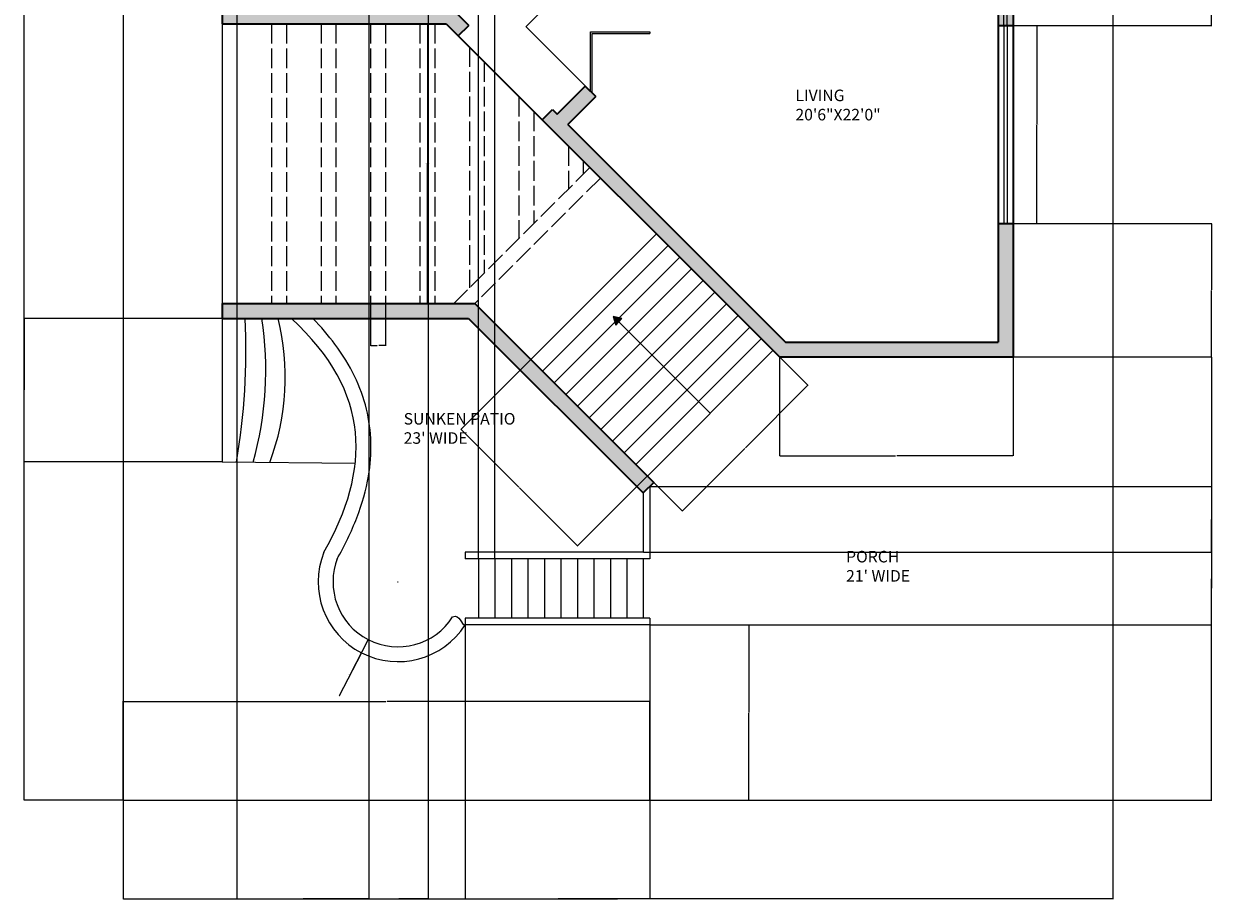
# Model space of a CAD drawing. Units: inches. Extents: x 1516 to 2236, y 3034 to 4235.
# Tile 1 of 3: x 1516 to 2236, y 3034 to 3566. Entities that reach past the tile are written whole.
import ezdxf

# ---------------------------------------------------------------- set-up
doc = ezdxf.new("R2010")
doc.units = ezdxf.units.IN
doc.linetypes.add('ACAD_ISO02W100', pattern=[15, 12, -3])
for name, color, linetype, lineweight in [('A-ANNO-DIMS', 2, 'Continuous', 18), ('A-ANNO-SYMB', 7, 'Continuous', 18), ('A-AREA-IDEN', 7, 'Continuous', 18), ('A-DOOR', 3, 'Continuous', 18), ('A-FLOR-STRS', 7, 'Continuous', 18), ('A-GLAZ', 4, 'Continuous', 18), ('A-ROOF-OVHD', 8, 'ACAD_ISO02W100', 18), ('A-WALL', 7, 'Continuous', 35), ('A-WALL-PATT', 252, 'Continuous', 13), ('C-PROP', 8, 'Continuous', 25), ('L-HRDS', 9, 'Continuous', 25)]:
    doc.layers.add(name, color=color, linetype=linetype, lineweight=lineweight)
doc.styles.get("Standard").update_dxf_attribs({"font": 'arial.ttf'})
doc.dimstyles.get("Standard").update_dxf_attribs({"dimtxt": 0.18, "dimasz": 0.18, "dimexe": 0.18, "dimexo": 0.0625, "dimgap": 0.09, "dimtad": 0, "dimtih": 1, "dimtoh": 1, "dimdec": 4, "dimzin": 0, "dimdsep": 46, "dimtxsty": 'Standard', "dimcen": 0.09, "dimadec": 0, "dimazin": 0, "dimtfac": 1, "dimtdec": 4, "dimtofl": 0, "dimtmove": 0, "dimatfit": 3, "dimfxl": 1, "dimtolj": 1, "dimtzin": 0, "dimarcsym": 0})

# ---------------------------------------------------------------- blocks, each defined once
blk = doc.blocks.new('WIN-120IN-GLASS')
for p, q in [((120, 2), (0, 2)), ((120, 0), (0, 0))]:
    blk.add_line(p, q)
blk = doc.blocks.new('TERRACE-OVHD-MEMBER')
for p, q in [((0, 169.71), (0, 0)), ((9, 169.71), (9, 0))]:
    blk.add_line(p, q)
blk = doc.blocks.new('*D10')
at = {"layer": 'A-ANNO-DIMS', "color": 0, "lineweight": -2, "transparency": 16777216}
for p, q in [((1735.08, 3565.52), (1760.65, 3565.52)), ((1760.47, 3565.34), (1760.47, 3480.85)), ((1760.47, 3396), (1760.47, 3480.49)), ((1735.08, 3395.82), (1760.65, 3395.82))]:
    blk.add_line(p, q, dxfattribs=at)
at = {"layer": 'A-ANNO-DIMS', "color": 0, "transparency": 16777216}
for points in [[(1760.44, 3565.34), (1760.5, 3565.34), (1760.47, 3565.52)], [(1760.44, 3396), (1760.5, 3396), (1760.47, 3395.82)]]:
    blk.add_solid(points, dxfattribs=at)
at = {"layer": 'Defpoints', "color": 0, "transparency": 16777216}
for p in [(1735.01, 3565.52), (1760.47, 3565.52), (1735.01, 3395.82)]:
    blk.add_point(p, dxfattribs=at)
at = {"layer": 'A-ANNO-DIMS', "color": 0, "transparency": 16777216, "insert": (1760.47, 3480.67), "char_height": 0.18, "attachment_point": 5}
blk.add_mtext('\\A1;OH MEMBER 170 TYP.', dxfattribs=at)
blk = doc.blocks.new('*D11')
at = {"layer": 'A-ANNO-DIMS', "color": 0, "lineweight": -2, "transparency": 16777216}
for p, q in [((1726.01, 3395.75), (1726.01, 3370.18)), ((1735.01, 3395.75), (1735.01, 3370.18)), ((1726.19, 3370.36), (1730.06, 3370.36)), ((1734.83, 3370.36), (1730.97, 3370.36))]:
    blk.add_line(p, q, dxfattribs=at)
at = {"layer": 'A-ANNO-DIMS', "color": 0, "transparency": 16777216}
for points in [[(1726.19, 3370.39), (1726.19, 3370.33), (1726.01, 3370.36)], [(1734.83, 3370.39), (1734.83, 3370.33), (1735.01, 3370.36)]]:
    blk.add_solid(points, dxfattribs=at)
at = {"layer": 'Defpoints', "color": 0, "transparency": 16777216}
for p in [(1726.01, 3395.82), (1735.01, 3395.82), (1735.01, 3370.36)]:
    blk.add_point(p, dxfattribs=at)
at = {"layer": 'A-ANNO-DIMS', "color": 0, "transparency": 16777216, "insert": (1730.51, 3370.36), "char_height": 0.18, "attachment_point": 5}
blk.add_mtext('\\A1;9 TYP.', dxfattribs=at)
blk = doc.blocks.new('*D12')
at = {"layer": 'A-ANNO-DIMS', "color": 0, "lineweight": -2, "transparency": 16777216}
for p, q in [((2112.08, 3564.41), (2130.19, 3564.41)), ((2130.01, 3564.23), (2130.01, 3504.59)), ((2130.01, 3444.59), (2130.01, 3504.23)), ((2112.08, 3444.41), (2130.19, 3444.41))]:
    blk.add_line(p, q, dxfattribs=at)
at = {"layer": 'A-ANNO-DIMS', "color": 0, "transparency": 16777216}
for points in [[(2129.98, 3564.23), (2130.04, 3564.23), (2130.01, 3564.41)], [(2129.98, 3444.59), (2130.04, 3444.59), (2130.01, 3444.41)]]:
    blk.add_solid(points, dxfattribs=at)
at = {"layer": 'Defpoints', "color": 0, "transparency": 16777216}
for p in [(2112.01, 3564.41), (2130.01, 3564.41), (2112.01, 3444.41)]:
    blk.add_point(p, dxfattribs=at)
at = {"layer": 'A-ANNO-DIMS', "color": 0, "transparency": 16777216, "insert": (2130.01, 3504.41), "char_height": 0.18, "attachment_point": 5}
blk.add_mtext('\\A1;WINDOW 120 TYP.', dxfattribs=at)
blk = doc.blocks.new('*D13')
at = {"layer": 'A-ANNO-DIMS', "color": 0, "lineweight": -2, "transparency": 16777216}
for p, q in [((2110.01, 3564.47), (2110.01, 3582.59)), ((2110.19, 3582.41), (2110.55, 3582.41)), ((2111.83, 3582.41), (2111.47, 3582.41)), ((2112.01, 3564.47), (2112.01, 3582.59))]:
    blk.add_line(p, q, dxfattribs=at)
at = {"layer": 'A-ANNO-DIMS', "color": 0, "transparency": 16777216}
for points in [[(2110.19, 3582.44), (2110.19, 3582.38), (2110.01, 3582.41)], [(2111.83, 3582.44), (2111.83, 3582.38), (2112.01, 3582.41)]]:
    blk.add_solid(points, dxfattribs=at)
at = {"layer": 'Defpoints', "color": 0, "transparency": 16777216}
for p in [(2110.01, 3582.41), (2110.01, 3564.41), (2112.01, 3564.41)]:
    blk.add_point(p, dxfattribs=at)
at = {"layer": 'A-ANNO-DIMS', "color": 0, "transparency": 16777216, "insert": (2111.01, 3582.41), "char_height": 0.18, "attachment_point": 5}
blk.add_mtext('\\A1;2 TYP.', dxfattribs=at)
blk = doc.blocks.new('*D16')
at = {"layer": 'A-ANNO-DIMS', "color": 0, "lineweight": -2, "transparency": 16777216}
for p, q in [((1576.01, 3094.46), (1576.01, 3034.44)), ((2176.01, 3094.46), (2176.01, 3034.44)), ((1576.19, 3034.62), (1875.73, 3034.62)), ((2175.83, 3034.62), (1876.3, 3034.62))]:
    blk.add_line(p, q, dxfattribs=at)
at = {"layer": 'A-ANNO-DIMS', "color": 0, "transparency": 16777216}
for points in [[(1576.19, 3034.65), (1576.19, 3034.59), (1576.01, 3034.62)], [(2175.83, 3034.65), (2175.83, 3034.59), (2176.01, 3034.62)]]:
    blk.add_solid(points, dxfattribs=at)
at = {"layer": 'Defpoints', "color": 0, "transparency": 16777216}
for p in [(1576.01, 3094.52), (2176.01, 3094.52), (1576.01, 3034.62)]:
    blk.add_point(p, dxfattribs=at)
at = {"layer": 'A-ANNO-DIMS', "color": 0, "transparency": 16777216, "insert": (1876.01, 3034.62), "char_height": 0.18, "attachment_point": 5}
blk.add_mtext('\\A1;600', dxfattribs=at)
blk = doc.blocks.new('*D17')
at = {"layer": 'A-ANNO-DIMS', "color": 0, "lineweight": -2, "transparency": 16777216}
for p, q in [((1575.95, 4174.52), (1515.93, 4174.52)), ((1516.11, 4174.34), (1516.11, 3634.7)), ((1516.11, 3094.7), (1516.11, 3634.34)), ((1575.95, 3094.52), (1515.93, 3094.52))]:
    blk.add_line(p, q, dxfattribs=at)
at = {"layer": 'A-ANNO-DIMS', "color": 0, "transparency": 16777216}
for points in [[(1516.08, 4174.34), (1516.14, 4174.34), (1516.11, 4174.52)], [(1516.08, 3094.7), (1516.14, 3094.7), (1516.11, 3094.52)]]:
    blk.add_solid(points, dxfattribs=at)
at = {"layer": 'Defpoints', "color": 0, "transparency": 16777216}
for p in [(1516.11, 4174.52), (1576.01, 4174.52), (1576.01, 3094.52)]:
    blk.add_point(p, dxfattribs=at)
at = {"layer": 'A-ANNO-DIMS', "color": 0, "transparency": 16777216, "insert": (1516.11, 3634.52), "char_height": 0.18, "attachment_point": 5}
blk.add_mtext('\\A1;1080', dxfattribs=at)
blk = doc.blocks.new('*D26')
at = {"layer": 'A-ANNO-DIMS', "color": 0, "lineweight": -2, "transparency": 16777216}
for p, q in [((2115.58, 3671.99), (2236.09, 3671.99)), ((2235.91, 3671.81), (2235.91, 3618.38)), ((2235.91, 3564.59), (2235.91, 3618.02)), ((2115.58, 3564.41), (2236.09, 3564.41))]:
    blk.add_line(p, q, dxfattribs=at)
at = {"layer": 'A-ANNO-DIMS', "color": 0, "transparency": 16777216}
for points in [[(2235.88, 3671.81), (2235.94, 3671.81), (2235.91, 3671.99)], [(2235.88, 3564.59), (2235.94, 3564.59), (2235.91, 3564.41)]]:
    blk.add_solid(points, dxfattribs=at)
at = {"layer": 'Defpoints', "color": 0, "transparency": 16777216}
for p in [(2115.51, 3671.99), (2235.91, 3671.99), (2115.51, 3564.41)]:
    blk.add_point(p, dxfattribs=at)
at = {"layer": 'A-ANNO-DIMS', "color": 0, "transparency": 16777216, "insert": (2235.91, 3618.2), "char_height": 0.18, "attachment_point": 5}
blk.add_mtext('\\A1;107.58', dxfattribs=at)
blk = doc.blocks.new('*D27')
at = {"layer": 'A-ANNO-DIMS', "color": 0, "lineweight": -2, "transparency": 16777216}
for p, q in [((2115.58, 3444.41), (2236.09, 3444.41)), ((2235.91, 3444.23), (2235.91, 3404.09)), ((2235.91, 3363.59), (2235.91, 3403.73)), ((2115.58, 3363.41), (2236.09, 3363.41))]:
    blk.add_line(p, q, dxfattribs=at)
at = {"layer": 'A-ANNO-DIMS', "color": 0, "transparency": 16777216}
for points in [[(2235.88, 3444.23), (2235.94, 3444.23), (2235.91, 3444.41)], [(2235.88, 3363.59), (2235.94, 3363.59), (2235.91, 3363.41)]]:
    blk.add_solid(points, dxfattribs=at)
at = {"layer": 'Defpoints', "color": 0, "transparency": 16777216}
for p in [(2115.51, 3444.41), (2235.91, 3444.41), (2115.51, 3363.41)]:
    blk.add_point(p, dxfattribs=at)
at = {"layer": 'A-ANNO-DIMS', "color": 0, "transparency": 16777216, "insert": (2235.91, 3403.91), "char_height": 0.18, "attachment_point": 5}
blk.add_mtext('\\A1;81', dxfattribs=at)
blk = doc.blocks.new('*D28')
at = {"layer": 'A-ANNO-DIMS', "color": 0, "lineweight": -2, "transparency": 16777216}
for p, q in [((2115.58, 3363.41), (2236.09, 3363.41)), ((2235.91, 3363.23), (2235.91, 3229.15)), ((2235.91, 3094.7), (2235.91, 3228.78)), ((2176.08, 3094.52), (2236.09, 3094.52))]:
    blk.add_line(p, q, dxfattribs=at)
at = {"layer": 'A-ANNO-DIMS', "color": 0, "transparency": 16777216}
for points in [[(2235.88, 3363.23), (2235.94, 3363.23), (2235.91, 3363.41)], [(2235.88, 3094.7), (2235.94, 3094.7), (2235.91, 3094.52)]]:
    blk.add_solid(points, dxfattribs=at)
at = {"layer": 'Defpoints', "color": 0, "transparency": 16777216}
for p in [(2115.51, 3363.41), (2235.91, 3363.41), (2176.01, 3094.52)]:
    blk.add_point(p, dxfattribs=at)
at = {"layer": 'A-ANNO-DIMS', "color": 0, "transparency": 16777216, "insert": (2235.91, 3228.97), "char_height": 0.18, "attachment_point": 5}
blk.add_mtext('\\A1;268.9', dxfattribs=at)
blk = doc.blocks.new('*D37')
at = {"layer": 'A-ANNO-DIMS', "color": 0, "lineweight": -2, "transparency": 16777216}
for p, q in [((1645.01, 3985.46), (1645.01, 3034.44)), ((1725.01, 3985.46), (1725.01, 3034.44)), ((1645.19, 3034.62), (1684.8, 3034.62)), ((1724.83, 3034.62), (1685.23, 3034.62))]:
    blk.add_line(p, q, dxfattribs=at)
at = {"layer": 'A-ANNO-DIMS', "color": 0, "transparency": 16777216}
for points in [[(1645.19, 3034.65), (1645.19, 3034.59), (1645.01, 3034.62)], [(1724.83, 3034.65), (1724.83, 3034.59), (1725.01, 3034.62)]]:
    blk.add_solid(points, dxfattribs=at)
at = {"layer": 'Defpoints', "color": 0, "transparency": 16777216}
for p in [(1645.01, 3985.52), (1725.01, 3985.52), (1725.01, 3034.62)]:
    blk.add_point(p, dxfattribs=at)
at = {"layer": 'A-ANNO-DIMS', "color": 0, "transparency": 16777216, "insert": (1685.01, 3034.62), "char_height": 0.18, "attachment_point": 5}
blk.add_mtext('\\A1;80', dxfattribs=at)
blk = doc.blocks.new('*D38')
at = {"layer": 'A-ANNO-DIMS', "color": 0, "lineweight": -2, "transparency": 16777216}
for p, q in [((1725.01, 3985.46), (1725.01, 3034.44)), ((1761.01, 3985.46), (1761.01, 3034.44)), ((1725.19, 3034.62), (1742.8, 3034.62)), ((1760.83, 3034.62), (1743.23, 3034.62))]:
    blk.add_line(p, q, dxfattribs=at)
at = {"layer": 'A-ANNO-DIMS', "color": 0, "transparency": 16777216}
for points in [[(1725.19, 3034.65), (1725.19, 3034.59), (1725.01, 3034.62)], [(1760.83, 3034.65), (1760.83, 3034.59), (1761.01, 3034.62)]]:
    blk.add_solid(points, dxfattribs=at)
at = {"layer": 'Defpoints', "color": 0, "transparency": 16777216}
for p in [(1725.01, 3985.52), (1761.01, 3985.52), (1761.01, 3034.62)]:
    blk.add_point(p, dxfattribs=at)
at = {"layer": 'A-ANNO-DIMS', "color": 0, "transparency": 16777216, "insert": (1743.01, 3034.62), "char_height": 0.18, "attachment_point": 5}
blk.add_mtext('\\A1;36', dxfattribs=at)
blk = doc.blocks.new('*D42')
at = {"layer": 'A-ANNO-DIMS', "color": 0, "lineweight": -2, "transparency": 16777216}
for p, q in [((1783.4, 3200.85), (1783.4, 3034.44)), ((1895.4, 3200.85), (1895.4, 3034.44)), ((1783.58, 3034.62), (1839.12, 3034.62)), ((1895.22, 3034.62), (1839.68, 3034.62))]:
    blk.add_line(p, q, dxfattribs=at)
at = {"layer": 'A-ANNO-DIMS', "color": 0, "transparency": 16777216}
for points in [[(1783.58, 3034.65), (1783.58, 3034.59), (1783.4, 3034.62)], [(1895.22, 3034.65), (1895.22, 3034.59), (1895.4, 3034.62)]]:
    blk.add_solid(points, dxfattribs=at)
at = {"layer": 'Defpoints', "color": 0, "transparency": 16777216}
for p in [(1783.4, 3200.91), (1895.4, 3200.91), (1895.4, 3034.62)]:
    blk.add_point(p, dxfattribs=at)
at = {"layer": 'A-ANNO-DIMS', "color": 0, "transparency": 16777216, "insert": (1839.4, 3034.62), "char_height": 0.18, "attachment_point": 5}
blk.add_mtext('\\A1;112', dxfattribs=at)
blk = doc.blocks.new('*D43')
at = {"layer": 'A-ANNO-DIMS', "color": 0, "lineweight": -2, "transparency": 16777216}
for p, q in [((1891.46332, 3244.909983), (2236.09429, 3244.909983)), ((2235.91429, 3244.729983), (2235.91429, 3223.089983)), ((2235.91429, 3201.089983), (2235.91429, 3222.729983)), ((1895.46332, 3200.909983), (2236.09429, 3200.909983))]:
    blk.add_line(p, q, dxfattribs=at)
at = {"layer": 'A-ANNO-DIMS', "color": 0, "transparency": 16777216}
for points in [[(2235.88429, 3244.729983), (2235.94429, 3244.729983), (2235.91429, 3244.909983)], [(2235.88429, 3201.089983), (2235.94429, 3201.089983), (2235.91429, 3200.909983)]]:
    blk.add_solid(points, dxfattribs=at)
at = {"layer": 'Defpoints', "color": 0, "transparency": 16777216}
for p in [(1891.40082, 3244.909983), (2235.91429, 3244.909983), (1895.40082, 3200.909983)]:
    blk.add_point(p, dxfattribs=at)
at = {"layer": 'A-ANNO-DIMS', "color": 0, "transparency": 16777216, "insert": (2235.91429, 3222.909983), "char_height": 0.18, "attachment_point": 5}
blk.add_mtext('\\A1;44', dxfattribs=at)
blk = doc.blocks.new('*D44')
at = {"layer": 'A-ANNO-DIMS', "color": 0, "lineweight": -2, "transparency": 16777216}
for p, q in [((1895.46, 3284.91), (2236.09, 3284.91)), ((2235.91, 3284.73), (2235.91, 3265.09)), ((2235.91, 3245.09), (2235.91, 3264.73)), ((1891.46, 3244.91), (2236.09, 3244.91))]:
    blk.add_line(p, q, dxfattribs=at)
at = {"layer": 'A-ANNO-DIMS', "color": 0, "transparency": 16777216}
for points in [[(2235.88, 3284.73), (2235.94, 3284.73), (2235.91, 3284.91)], [(2235.88, 3245.09), (2235.94, 3245.09), (2235.91, 3244.91)]]:
    blk.add_solid(points, dxfattribs=at)
at = {"layer": 'Defpoints', "color": 0, "transparency": 16777216}
for p in [(1895.4, 3284.91), (2235.91, 3284.91), (1891.4, 3244.91)]:
    blk.add_point(p, dxfattribs=at)
at = {"layer": 'A-ANNO-DIMS', "color": 0, "transparency": 16777216, "insert": (2235.91, 3264.91), "char_height": 0.18, "attachment_point": 5}
blk.add_mtext('\\A1;40', dxfattribs=at)
blk = doc.blocks.new('*D45')
at = {"layer": 'A-ANNO-DIMS', "color": 0, "lineweight": -2, "transparency": 16777216}
for p, q in [((1635.95, 3386.82), (1515.93, 3386.82)), ((1516.11, 3386.64), (1516.11, 3343.44)), ((1516.11, 3299.88), (1516.11, 3343.08)), ((1635.95, 3299.7), (1515.93, 3299.7))]:
    blk.add_line(p, q, dxfattribs=at)
at = {"layer": 'A-ANNO-DIMS', "color": 0, "transparency": 16777216}
for points in [[(1516.08, 3386.64), (1516.14, 3386.64), (1516.11, 3386.82)], [(1516.08, 3299.88), (1516.14, 3299.88), (1516.11, 3299.7)]]:
    blk.add_solid(points, dxfattribs=at)
at = {"layer": 'Defpoints', "color": 0, "transparency": 16777216}
for p in [(1636.01, 3386.82), (1516.11, 3299.7), (1636.01, 3299.7)]:
    blk.add_point(p, dxfattribs=at)
at = {"layer": 'A-ANNO-DIMS', "color": 0, "transparency": 16777216, "insert": (1516.11, 3343.26), "char_height": 0.18, "attachment_point": 5}
blk.add_mtext('\\A1;87.11', dxfattribs=at)
blk = doc.blocks.new('*D46')
at = {"layer": 'A-ANNO-DIMS', "color": 0, "lineweight": -2, "transparency": 16777216}
for p, q in [((1576.01, 3094.58), (1576.01, 3154.6)), ((1576.19, 3154.42), (1735.31, 3154.42)), ((1895.22, 3154.42), (1736.1, 3154.42)), ((1895.4, 3094.58), (1895.4, 3154.6))]:
    blk.add_line(p, q, dxfattribs=at)
at = {"layer": 'A-ANNO-DIMS', "color": 0, "transparency": 16777216}
for points in [[(1576.19, 3154.45), (1576.19, 3154.39), (1576.01, 3154.42)], [(1895.22, 3154.45), (1895.22, 3154.39), (1895.4, 3154.42)]]:
    blk.add_solid(points, dxfattribs=at)
at = {"layer": 'Defpoints', "color": 0, "transparency": 16777216}
for p in [(1895.4, 3154.42), (1576.01, 3094.52), (1895.4, 3094.52)]:
    blk.add_point(p, dxfattribs=at)
at = {"layer": 'A-ANNO-DIMS', "color": 0, "transparency": 16777216, "insert": (1735.71, 3154.42), "char_height": 0.18, "attachment_point": 5}
blk.add_mtext('\\A1;319.4', dxfattribs=at)
blk = doc.blocks.new('*D47')
at = {"layer": 'A-ANNO-DIMS', "color": 0, "lineweight": -2, "transparency": 16777216}
for p, q in [((1948.84, 3388.47), (1991.28, 3346.03)), ((1991.03, 3346.03), (1953.27, 3308.27)), ((1872.71, 3312.33), (1915.15, 3269.89)), ((1915.15, 3270.15), (1952.9, 3307.91))]:
    blk.add_line(p, q, dxfattribs=at)
at = {"layer": 'A-ANNO-DIMS', "color": 0, "transparency": 16777216}
for points in [[(1991.01, 3346.05), (1991.05, 3346.01), (1991.15, 3346.16)], [(1915.12, 3270.17), (1915.17, 3270.13), (1915.02, 3270.02)]]:
    blk.add_solid(points, dxfattribs=at)
at = {"layer": 'Defpoints', "color": 0, "transparency": 16777216}
for p in [(1948.8, 3388.51), (1872.66, 3312.38), (1915.02, 3270.02)]:
    blk.add_point(p, dxfattribs=at)
at = {"layer": 'A-ANNO-DIMS', "color": 0, "transparency": 16777216, "insert": (1953.09, 3308.09), "char_height": 0.18, "attachment_point": 5}
blk.add_mtext('\\A1;107.67', dxfattribs=at)
blk = doc.blocks.new('*D48')
at = {"layer": 'A-ANNO-DIMS', "color": 0, "lineweight": -2, "transparency": 16777216}
for p, q in [((1823.12, 3361.83), (1780.68, 3319.39)), ((1780.94, 3319.39), (1815.98, 3284.34)), ((1893.83, 3291.12), (1851.39, 3248.68)), ((1851.39, 3248.93), (1816.35, 3283.98))]:
    blk.add_line(p, q, dxfattribs=at)
at = {"layer": 'A-ANNO-DIMS', "color": 0, "transparency": 16777216}
for points in [[(1780.96, 3319.41), (1780.92, 3319.37), (1780.81, 3319.52)], [(1851.41, 3248.96), (1851.37, 3248.91), (1851.52, 3248.81)]]:
    blk.add_solid(points, dxfattribs=at)
at = {"layer": 'Defpoints', "color": 0, "transparency": 16777216}
for p in [(1823.16, 3361.87), (1780.81, 3319.52), (1893.88, 3291.16)]:
    blk.add_point(p, dxfattribs=at)
at = {"layer": 'A-ANNO-DIMS', "color": 0, "transparency": 16777216, "insert": (1816.16, 3284.16), "char_height": 0.18, "attachment_point": 5}
blk.add_mtext('\\A1;100', dxfattribs=at)
blk = doc.blocks.new('*D49')
at = {"layer": 'A-ANNO-DIMS', "color": 0, "lineweight": -2, "transparency": 16777216}
for p, q in [((1791.4, 3240.97), (1791.4, 4234.6)), ((1791.58, 4234.42), (1796.19, 4234.42)), ((1801.22, 4234.42), (1796.61, 4234.42)), ((1801.4, 3240.97), (1801.4, 4234.6))]:
    blk.add_line(p, q, dxfattribs=at)
at = {"layer": 'A-ANNO-DIMS', "color": 0, "transparency": 16777216}
for points in [[(1791.58, 4234.45), (1791.58, 4234.39), (1791.4, 4234.42)], [(1801.22, 4234.45), (1801.22, 4234.39), (1801.4, 4234.42)]]:
    blk.add_solid(points, dxfattribs=at)
at = {"layer": 'Defpoints', "color": 0, "transparency": 16777216}
for p in [(1801.4, 4234.42), (1791.4, 3240.91), (1801.4, 3240.91)]:
    blk.add_point(p, dxfattribs=at)
at = {"layer": 'A-ANNO-DIMS', "color": 0, "transparency": 16777216, "insert": (1796.4, 4234.42), "char_height": 0.18, "attachment_point": 5}
blk.add_mtext('\\A1;10', dxfattribs=at)
blk = doc.blocks.new('*D56')
at = {"layer": 'A-ANNO-DIMS', "color": 0, "lineweight": -2, "transparency": 16777216}
for p, q in [((1973.9, 3363.35), (1973.9, 3303.33)), ((2115.51, 3363.35), (2115.51, 3303.33)), ((1974.08, 3303.51), (2044.32, 3303.51)), ((2115.33, 3303.51), (2045.09, 3303.51))]:
    blk.add_line(p, q, dxfattribs=at)
at = {"layer": 'A-ANNO-DIMS', "color": 0, "transparency": 16777216}
for points in [[(1974.08, 3303.54), (1974.08, 3303.48), (1973.9, 3303.51)], [(2115.33, 3303.54), (2115.33, 3303.48), (2115.51, 3303.51)]]:
    blk.add_solid(points, dxfattribs=at)
at = {"layer": 'Defpoints', "color": 0, "transparency": 16777216}
for p in [(1973.9, 3363.41), (2115.51, 3363.41), (1973.9, 3303.51)]:
    blk.add_point(p, dxfattribs=at)
at = {"layer": 'A-ANNO-DIMS', "color": 0, "transparency": 16777216, "insert": (2044.71, 3303.51), "char_height": 0.18, "attachment_point": 5}
blk.add_mtext('\\A1;141.6', dxfattribs=at)
blk = doc.blocks.new('*D57')
at = {"layer": 'A-ANNO-DIMS', "color": 0, "lineweight": -2, "transparency": 16777216}
for p, q in [((1895.46, 3200.91), (1955.48, 3200.91)), ((1955.3, 3200.73), (1955.3, 3147.9)), ((1955.3, 3094.7), (1955.3, 3147.53)), ((1895.46, 3094.52), (1955.48, 3094.52))]:
    blk.add_line(p, q, dxfattribs=at)
at = {"layer": 'A-ANNO-DIMS', "color": 0, "transparency": 16777216}
for points in [[(1955.27, 3200.73), (1955.33, 3200.73), (1955.3, 3200.91)], [(1955.27, 3094.7), (1955.33, 3094.7), (1955.3, 3094.52)]]:
    blk.add_solid(points, dxfattribs=at)
at = {"layer": 'Defpoints', "color": 0, "transparency": 16777216}
for p in [(1895.4, 3200.91), (1895.4, 3094.52), (1955.3, 3094.52)]:
    blk.add_point(p, dxfattribs=at)
at = {"layer": 'A-ANNO-DIMS', "color": 0, "transparency": 16777216, "insert": (1955.3, 3147.72), "char_height": 0.18, "attachment_point": 5}
blk.add_mtext('\\A1;106.39', dxfattribs=at)
blk = doc.blocks.new('*D60')
at = {"layer": 'A-ANNO-DIMS', "color": 0, "lineweight": -2, "transparency": 16777216}
for p, q in [((1918.17, 3661.67), (1869.45, 3612.95)), ((1960.61, 3619.48), (1918.17, 3661.92)), ((1820.37, 3563.86), (1869.09, 3612.58)), ((1862.55, 3521.42), (1820.12, 3563.86))]:
    blk.add_line(p, q, dxfattribs=at)
at = {"layer": 'A-ANNO-DIMS', "color": 0, "transparency": 16777216}
for points in [[(1918.15, 3661.69), (1918.2, 3661.65), (1918.3, 3661.79)], [(1820.35, 3563.88), (1820.39, 3563.84), (1820.24, 3563.74)]]:
    blk.add_solid(points, dxfattribs=at)
at = {"layer": 'Defpoints', "color": 0, "transparency": 16777216}
for p in [(1918.3, 3661.79), (1960.66, 3619.44), (1862.6, 3521.38)]:
    blk.add_point(p, dxfattribs=at)
at = {"layer": 'A-ANNO-DIMS', "color": 0, "transparency": 16777216, "insert": (1869.27, 3612.77), "char_height": 0.18, "attachment_point": 5}
blk.add_mtext('\\A1;138.68', dxfattribs=at)
blk = doc.blocks.new('*D61')
at = {"layer": 'A-ANNO-DIMS', "color": 0, "lineweight": -2, "transparency": 16777216}
for p, q in [((1742.55, 3226.94), (1742.73, 3226.94)), ((1742.64, 3226.85), (1742.64, 3227.03)), ((1707.29, 3158.11), (1720.46, 3183.76)), ((1707.11, 3158.11), (1707.29, 3158.11))]:
    blk.add_line(p, q, dxfattribs=at)
at = {"layer": 'A-ANNO-DIMS', "color": 0, "transparency": 16777216}
blk.add_solid([(1720.44, 3183.78), (1720.49, 3183.75), (1720.54, 3183.92)], dxfattribs=at)
at = {"layer": 'Defpoints', "color": 0, "transparency": 16777216}
for p in [(1742.64, 3226.94), (1720.54, 3183.92)]:
    blk.add_point(p, dxfattribs=at)
at = {"layer": 'A-ANNO-DIMS', "color": 0, "transparency": 16777216, "insert": (1706.63, 3158.11), "char_height": 0.18, "attachment_point": 5}
blk.add_mtext('\\A1;R48.36', dxfattribs=at)
blk = doc.blocks.new('*D62')
at = {"layer": 'A-ANNO-DIMS', "color": 0, "lineweight": -2, "transparency": 16777216}
for p, q in [((1742.55, 3226.94), (1742.73, 3226.94)), ((1742.64, 3226.85), (1742.64, 3227.03)), ((1713.87, 3170.92), (1724.57, 3191.77)), ((1713.69, 3170.92), (1713.87, 3170.92))]:
    blk.add_line(p, q, dxfattribs=at)
at = {"layer": 'A-ANNO-DIMS', "color": 0, "transparency": 16777216}
blk.add_solid([(1724.55, 3191.78), (1724.6, 3191.75), (1724.66, 3191.93)], dxfattribs=at)
at = {"layer": 'Defpoints', "color": 0, "transparency": 16777216}
for p in [(1742.64, 3226.94), (1724.66, 3191.93)]:
    blk.add_point(p, dxfattribs=at)
at = {"layer": 'A-ANNO-DIMS', "color": 0, "transparency": 16777216, "insert": (1713.21, 3170.92), "char_height": 0.18, "attachment_point": 5}
blk.add_mtext('\\A1;R39.36', dxfattribs=at)

msp = doc.modelspace()

# ---------------------------------------------------------------- hatches: boundary and pattern name
at = {"layer": 'A-ANNO-SYMB'}
h = msp.add_hatch(color=256, dxfattribs=at)
h.dxf.hatch_style = 1
h.paths.add_polyline_path([(1878.3495, 3386.7438), (1873.0698, 3387.9039), (1874.705, 3382.7515)])
at = {"layer": 'A-WALL-PATT'}
h = msp.add_hatch(color=256, dxfattribs=at)
h.dxf.hatch_style = 1
h.paths.add_polyline_path([(2115.5143, 3444.4097), (2106.5143, 3444.4097), (2106.5143, 3372.4097), (1977.6285, 3372.4097), (1845.6285, 3504.4097), (1862.599, 3521.3803), (1856.2351, 3527.7442), (1839.2645, 3510.7737), (1836.4361, 3513.6021), (1830.0721, 3507.2381), (1973.9005, 3363.4097), (2115.5143, 3363.4097)])
h.paths.add_polyline_path([(2115.5143, 3671.9887), (2106.5143, 3671.9887), (2106.5143, 3645.4097), (1981.3564, 3645.4097), (1963.6205, 3663.1456), (1957.2565, 3656.7817), (1971.2645, 3642.7737), (1954.2939, 3625.8031), (1960.6579, 3619.4391), (1977.6285, 3636.4097), (2106.5143, 3636.4097), (2106.5143, 3564.4097), (2115.5143, 3564.4097)])
h.paths.add_polyline_path([(1975.583, 3914.2268), (1978.4114, 3917.0552), (1972.0475, 3923.4192), (1951.7986, 3903.1703), (1958.1625, 3896.8063), (1969.219, 3907.8629), (2030.7373, 3846.3446), (1905.5794, 3721.1867), (1901.3368, 3725.4293), (1894.9728, 3719.0653), (1923.3154, 3690.7228), (1929.6793, 3697.0868), (1911.9434, 3714.8227), (2037.1013, 3839.9806), (2106.5143, 3770.5676), (2106.5143, 3743.9887), (2115.5143, 3743.9887), (2115.5143, 3774.2955), (2056.9238, 3832.886), (2115.5143, 3891.4765), (2115.5143, 3928.3632), (2106.5143, 3928.3632), (2106.5143, 3895.2044), (2050.5598, 3839.25)])
h.paths.add_polyline_path([(1806.5143, 3991.886), (1806.5143, 4105.5221), (1863.5143, 4105.5221), (1863.5143, 4114.5221), (1771.2643, 4114.5221), (1771.2643, 4105.5221), (1797.5143, 4105.5221), (1797.5143, 3994.5221), (1761.0143, 3994.5221), (1761.0143, 3985.5221), (1800.1503, 3985.5221), (1917.1503, 3868.5221), (1914.3219, 3865.6936), (1920.6859, 3859.3297), (1923.5143, 3862.1581), (1932.7067, 3871.3505), (1926.3427, 3877.7144), (1923.5143, 3874.886)])
h.paths.add_polyline_path([(1895.23, 3833.8738), (1888.8661, 3840.2378), (1812.1503, 3763.5221), (1645.0143, 3763.5221), (1645.0143, 3814.5221), (1636.0143, 3814.5221), (1636.0143, 3565.5221), (1771.7882, 3565.5221), (1779.1604, 3558.1498), (1785.5244, 3564.5138), (1775.5161, 3574.5221), (1645.0143, 3574.5221), (1645.0143, 3754.5221), (1815.8783, 3754.5221), (1837.6972, 3776.341), (1841.9398, 3772.0983), (1848.3038, 3778.4623), (1844.0611, 3782.7049)])
h.paths.add_polyline_path([(1645.0143, 3985.5221), (1725.0143, 3985.5221), (1725.0143, 3994.5221), (1721.0143, 3994.5221), (1721.0143, 3998.5221), (1717.0143, 3998.5221), (1717.0143, 3994.5221), (1645.0143, 3994.5221), (1645.0143, 4105.5221), (1669.0143, 4105.5221), (1669.0143, 4114.5221), (1636.0143, 4114.5221), (1636.0143, 3934.5221), (1645.0143, 3934.5221)])
h.paths.add_polyline_path([(1747.2643, 4114.5221), (1693.0143, 4114.5221), (1693.0143, 4105.5221), (1717.0143, 4105.5221), (1717.0143, 4028.5221), (1721.0143, 4028.5221), (1721.0143, 4041.5221), (1725.0143, 4041.5221), (1725.0143, 4045.5221), (1721.0143, 4045.5221), (1721.0143, 4105.5221), (1747.2643, 4105.5221)])
h.paths.add_polyline_path([(2066.0143, 4114.5221), (1983.5143, 4114.5221), (1983.5143, 4105.5221), (2040.5143, 4105.5221), (2040.5143, 4068.0221), (2049.5143, 4068.0221), (2049.5143, 4105.5221), (2066.0143, 4105.5221)])
h.paths.add_polyline_path([(2115.5143, 4114.5221), (2090.0143, 4114.5221), (2090.0143, 4105.5221), (2106.5143, 4105.5221), (2106.5143, 3994.5221), (2049.5143, 3994.5221), (2049.5143, 4032.0221), (2040.5143, 4032.0221), (2040.5143, 3991.886), (1997.5033, 3948.875), (2003.8673, 3942.5111), (2046.8783, 3985.5221), (2106.5143, 3985.5221), (2106.5143, 3952.3632), (2115.5143, 3952.3632)])
h.paths.add_polyline_path([(1789.2236, 3395.8151), (1636.0143, 3395.8151), (1636.0143, 3386.8151), (1785.4957, 3386.8151), (1891.4008, 3280.91), (1897.7648, 3287.2739)])

# ---------------------------------------------------------------- linework, layer by layer
at = {"layer": 'A-ANNO-SYMB'}
msp.add_line((1931.9433, 3329.2312), (1876.4793, 3384.6952), dxfattribs=at)
msp.add_lwpolyline([(1873.0698, 3387.9039), (1874.705, 3382.7515), (1878.3495, 3386.7438)], close=True, dxfattribs=at)
at = {"layer": 'A-DOOR'}
for p, q in [((1859.417, 3524.5623), (1859.417, 3560.5623)), ((1859.417, 3560.5623), (1895.417, 3560.5623)), ((1860.417, 3523.5623), (1860.417, 3559.5623)), ((1860.417, 3559.5623), (1895.417, 3559.5623)), ((1895.417, 3560.5623), (1895.417, 3559.5623))]:
    msp.add_line(p, q, dxfattribs=at)
at = {"layer": 'A-FLOR-STRS'}
for p, q in [((1899.3005, 3438.0098), (1823.1647, 3361.874)), ((1906.3716, 3430.9387), (1830.2358, 3354.8029)), ((1913.4426, 3423.8676), (1876.6846, 3387.1096)), ((1920.5137, 3416.7965), (1844.3779, 3340.6608)), ((1927.5848, 3409.7255), (1851.449, 3333.5897)), ((1934.6558, 3402.6544), (1858.5201, 3326.5186)), ((1941.7269, 3395.5833), (1865.5911, 3319.4476)), ((1948.798, 3388.5123), (1872.6622, 3312.3765)), ((1874.132, 3384.557), (1837.3069, 3347.7319)), ((1955.869, 3381.4412), (1879.7333, 3305.3054)), ((1962.9401, 3374.3701), (1886.8043, 3298.2344)), ((1970.0112, 3367.2991), (1893.8754, 3291.1633)), ((1791.4008, 3240.91), (1791.4008, 3204.91)), ((1801.4008, 3240.91), (1801.4008, 3204.91)), ((1811.4008, 3240.91), (1811.4008, 3204.91)), ((1821.4008, 3240.91), (1821.4008, 3204.91)), ((1831.4008, 3240.91), (1831.4008, 3204.91)), ((1841.4008, 3240.91), (1841.4008, 3204.91)), ((1851.4008, 3240.91), (1851.4008, 3204.91)), ((1861.4008, 3240.91), (1861.4008, 3204.91)), ((1861.4008, 3240.91), (1861.4008, 3204.91)), ((1871.4008, 3240.91), (1871.4008, 3204.91)), ((1881.4008, 3240.91), (1881.4008, 3204.91)), ((1891.4008, 3240.91), (1891.4008, 3204.91))]:
    msp.add_line(p, q, dxfattribs=at)
at = {"layer": 'A-ROOF-OVHD'}
for p, q in [((1645.0143, 3565.5221), (1645.0143, 3395.8151)), ((1786.0143, 3551.296), (1786.0143, 3405.3337)), ((1795.0143, 3542.296), (1795.0143, 3414.3337)), ((1816.0143, 3521.296), (1816.0143, 3435.3337)), ((1825.0143, 3512.296), (1825.0143, 3444.3337)), ((1846.0143, 3491.296), (1846.0143, 3465.3337)), ((1855.0143, 3482.296), (1855.0143, 3474.3337)), ((1858.9954, 3478.3148), (1776.4957, 3395.8151)), ((1865.3594, 3471.9509), (1789.2236, 3395.8151))]:
    msp.add_line(p, q, dxfattribs=at)
at = {"layer": 'A-WALL'}
for p, q in [((1636.0143, 4114.5221), (1636.0143, 3565.5221)), ((2115.5143, 3774.2955), (2115.5143, 3363.4097)), ((2106.5143, 3636.4097), (2106.5143, 3372.4097)), ((1775.5161, 3574.5221), (1785.5244, 3564.5138)), ((1636.0143, 3565.5221), (1771.7882, 3565.5221)), ((1771.7882, 3565.5221), (1779.1604, 3558.1498)), ((1779.1604, 3558.1498), (1785.5244, 3564.5138)), ((2106.5143, 3564.4097), (2115.5143, 3564.4097)), ((1779.1604, 3558.1498), (1973.9005, 3363.4097)), ((1839.2645, 3510.7737), (1856.2351, 3527.7442)), ((1856.2351, 3527.7442), (1862.599, 3521.3803)), ((1845.6285, 3504.4097), (1862.599, 3521.3803)), ((1830.0721, 3507.2381), (1836.4361, 3513.6021)), ((1836.4361, 3513.6021), (1839.2645, 3510.7737)), ((1845.6285, 3504.4097), (1977.6285, 3372.4097)), ((2106.5143, 3444.4097), (2115.5143, 3444.4097)), ((1636.0143, 3395.8151), (1789.2236, 3395.8151)), ((1636.0143, 3395.8151), (1636.0143, 3386.8151)), ((1789.2236, 3395.8151), (1897.7648, 3287.2739)), ((1636.0143, 3386.8151), (1785.4957, 3386.8151)), ((1785.4957, 3386.8151), (1891.4008, 3280.91)), ((1977.6285, 3372.4097), (2106.5143, 3372.4097)), ((1973.9005, 3363.4097), (2115.5143, 3363.4097)), ((1897.7648, 3287.2739), (1891.4008, 3280.91))]:
    msp.add_line(p, q, dxfattribs=at)
at = {"layer": 'C-PROP'}
for p, q in [((1576.0143, 4174.5221), (1576.0143, 3094.5221)), ((2176.0143, 4174.5221), (2176.0143, 3094.5221)), ((1576.0143, 3094.5221), (2176.0143, 3094.5221))]:
    msp.add_line(p, q, dxfattribs=at)
at = {"layer": 'L-HRDS'}
for p, q in [((1636.0143, 3565.5221), (1636.0143, 3395.8151)), ((1636.0143, 3386.8151), (1636.0143, 3299.7017)), ((1636.0143, 3299.7017), (1716.765, 3299.0445)), ((1891.4008, 3280.91), (1891.4008, 3244.91)), ((1895.4008, 3284.91), (1895.4008, 3240.91)), ((1891.4008, 3244.91), (1783.4008, 3244.91)), ((1783.4008, 3244.91), (1783.4008, 3240.91)), ((1895.4008, 3240.91), (1783.4008, 3240.91)), ((1895.4008, 3204.91), (1783.4008, 3204.91)), ((1783.4008, 3204.91), (1783.4008, 3200.91)), ((1895.4008, 3200.91), (1783.4008, 3200.91)), ((1895.4008, 3204.91), (1895.4008, 3094.5221))]:
    msp.add_line(p, q, dxfattribs=at)
for centre, radius, start, end in [((1247.967, 3367.4815), 402.5489, 350.2962926, 2.7528661), ((1456.7848, 3355.0904), 205.7385, 344.3378111, 8.8703685), ((1525.7195, 3351.368), 148.6423, 339.5631238, 13.7964222), ((1742.642, 3226.9394), 48.3613, 158.1862676, 327.4368924), ((1742.642, 3226.9394), 39.3613, 158.1862676, 327.4368924)]:
    msp.add_arc(centre, radius, start, end, dxfattribs=at)
for points in [[(1697.7435, 3244.91), (1726.1422, 3295.366), (1726.8535, 3341.4676), (1678.1212, 3386.8151)], [(1775.8156, 3205.754), (1780.4242, 3207.8981), (1780.8568, 3200.3358), (1783.4008, 3200.91)]]:
    msp.add_open_spline(points, degree=3, dxfattribs=at)
msp.add_open_spline([(1705.5865, 3240.4956), (1710.3648, 3248.9852), (1714.4309, 3257.4279), (1720.9061, 3274.2953), (1723.315, 3282.7227), (1725.9134, 3297.9572), (1726.441, 3304.7614), (1726.0832, 3318.3372), (1725.1964, 3325.1073), (1721.9066, 3338.5288), (1719.5046, 3345.1779), (1713.1454, 3358.2933), (1709.19, 3364.7596), (1700.5101, 3376.4195), (1696.0333, 3381.6424), (1690.9979, 3386.8151)], degree=3, knots=[0, 0, 0, 0, 26.39404101, 26.39404101, 52.78808201, 52.78808201, 74.063542, 74.063542, 95.33900199, 95.33900199, 116.61446198, 116.61446198, 137.88992197, 137.88992197, 155.52498749, 155.52498749, 155.52498749, 155.52498749], dxfattribs=at)

# ---------------------------------------------------------------- block references
at = {"layer": 'A-GLAZ', "rotation": 89.9999999999983}
msp.add_blockref('WIN-120IN-GLASS', (2112.0143, 3444.4097), dxfattribs=at)
at = {"layer": 'A-ROOF-OVHD'}
for p in [(1666.0143, 3395.8151), (1696.0143, 3395.8151), (1726.0143, 3395.8151), (1756.0143, 3395.8151)]:
    msp.add_blockref('TERRACE-OVHD-MEMBER', p, dxfattribs=at)

# ---------------------------------------------------------------- texts
at = {"layer": 'A-AREA-IDEN', "char_height": 7, "attachment_point": 1}
for s, width, insert in [('LIVING\\P20\'6"X22\'0"', 47.692137, (1983.6229, 3525.5701)), ("SUNKEN PATIO\\P23' WIDE", 111.980869, (1746.109, 3329.3813)), ("PORCH\\P21' WIDE", 47.692137, (2014.3384, 3245.7643))]:
    msp.add_mtext_dynamic_manual_height_columns(s, width=width, gutter_width=12.5, heights=[0], dxfattribs=dict(at, insert=insert))

# ---------------------------------------------------------------- dimensions: what is measured, and where the dimension line sits
at = {"layer": 'A-ANNO-DIMS'}
for base, p1, p2, override, picture, middle in [((1801.4008, 4234.4221), (1791.4008, 3240.91), (1801.4008, 3240.91), {"dimdec": 0, "dimlfac": 1, "dimrnd": 0, "dimzin": 0, "dimdsep": 46, "dimlunit": 2}, '*D49', (1796.4008, 4234.4221)), ((1725.0143, 3034.6221), (1645.0143, 3985.5221), (1725.0143, 3985.5221), {"dimdec": 0, "dimlfac": 1, "dimrnd": 0, "dimzin": 0, "dimdsep": 46, "dimlunit": 2}, '*D37', (1685.0143, 3034.6221)), ((1761.0143, 3034.6221), (1725.0143, 3985.5221), (1761.0143, 3985.5221), {"dimdec": 0, "dimlfac": 1, "dimrnd": 0, "dimzin": 0, "dimdsep": 46, "dimlunit": 2}, '*D38', (1743.0143, 3034.6221)), ((1895.4008, 3034.6221), (1783.4008, 3200.91), (1895.4008, 3200.91), {"dimdec": 0, "dimlfac": 1, "dimrnd": 0, "dimzin": 0, "dimdsep": 46, "dimlunit": 2}, '*D42', (1839.4008, 3034.6221)), ((1895.4008, 3154.4221), (1576.0143, 3094.5221), (1895.4008, 3094.5221), {"dimdec": 1, "dimlfac": 1, "dimrnd": 0, "dimzin": 0, "dimdsep": 46, "dimlunit": 2}, '*D46', (1735.7076, 3154.4221))]:
    dim = msp.add_linear_dim(base=base, p1=p1, p2=p2, dimstyle='Standard', override=override, dxfattribs=at)
    dim.commit()
    dim.dimension.update_dxf_attribs({"geometry": picture, "text_midpoint": middle})
for base, p1, p2, angle, override, picture, middle in [((1516.1143, 4174.5221), (1576.0143, 3094.5221), (1576.0143, 4174.5221), 90, {"dimdec": 0, "dimlfac": 1, "dimrnd": 0, "dimzin": 0, "dimdsep": 46, "dimlunit": 2}, '*D17', (1516.1143, 3634.5221)), ((2235.9143, 3671.9887), (2115.5143, 3564.4097), (2115.5143, 3671.9887), 90, {"dimdec": 2, "dimlfac": 1, "dimrnd": 0, "dimzin": 0, "dimdsep": 46, "dimlunit": 2}, '*D26', (2235.9143, 3618.1992)), ((1918.3022, 3661.7948), (1862.599, 3521.3803), (1960.6579, 3619.4391), 45, {"dimdec": 2, "dimlfac": 1, "dimrnd": 0, "dimzin": 0, "dimdsep": 46, "dimlunit": 2}, '*D60', (1869.2728, 3612.7654)), ((2235.9143, 3444.4097), (2115.5143, 3363.4097), (2115.5143, 3444.4097), 90, {"dimdec": 0, "dimlfac": 1, "dimrnd": 0, "dimzin": 0, "dimdsep": 46, "dimlunit": 2}, '*D27', (2235.9143, 3403.9097)), ((1516.1143, 3299.7017), (1636.0143, 3386.8151), (1636.0143, 3299.7017), 90, {"dimdec": 2, "dimlfac": 1, "dimrnd": 0, "dimzin": 0, "dimdsep": 46, "dimlunit": 2}, '*D45', (1516.1143, 3343.2584)), ((1915.0179, 3270.0208), (1948.798, 3388.5123), (1872.6622, 3312.3765), 225, {"dimdec": 2, "dimlfac": 1, "dimrnd": 0, "dimzin": 0, "dimdsep": 46, "dimlunit": 2}, '*D47', (1953.0858, 3308.0887)), ((1780.809, 3319.5183), (1893.8754, 3291.1633), (1823.1647, 3361.874), 135, {"dimdec": 0, "dimlfac": 1, "dimrnd": 0, "dimzin": 0, "dimdsep": 46, "dimlunit": 2}, '*D48', (1816.1644, 3284.163)), ((1973.9005, 3303.5097), (2115.5143, 3363.4097), (1973.9005, 3363.4097), 180, {"dimdec": 1, "dimlfac": 1, "dimrnd": 0, "dimzin": 0, "dimdsep": 46, "dimlunit": 2}, '*D56', (2044.7074, 3303.5097)), ((2235.9143, 3363.4097), (2176.0143, 3094.5221), (2115.5143, 3363.4097), 90, {"dimdec": 1, "dimlfac": 1, "dimrnd": 0, "dimzin": 0, "dimdsep": 46, "dimlunit": 2}, '*D28', (2235.9143, 3228.9659)), ((2235.9143, 3284.91), (1891.4008, 3244.91), (1895.4008, 3284.91), 90, {"dimdec": 0, "dimlfac": 1, "dimrnd": 0, "dimzin": 0, "dimdsep": 46, "dimlunit": 2}, '*D44', (2235.9143, 3264.91)), ((2235.9143, 3244.91), (1895.4008, 3200.91), (1891.4008, 3244.91), 90, {"dimdec": 0, "dimlfac": 1, "dimrnd": 0, "dimzin": 0, "dimdsep": 46, "dimlunit": 2}, '*D43', (2235.9143, 3222.91)), ((1955.3008, 3094.5221), (1895.4008, 3200.91), (1895.4008, 3094.5221), 270, {"dimdec": 2, "dimlfac": 1, "dimrnd": 0, "dimzin": 0, "dimdsep": 46, "dimlunit": 2}, '*D57', (1955.3008, 3147.716)), ((1576.0143, 3034.6221), (2176.0143, 3094.5221), (1576.0143, 3094.5221), 180, {"dimdec": 0, "dimlfac": 1, "dimrnd": 0, "dimzin": 0, "dimdsep": 46, "dimlunit": 2}, '*D16', (1876.0143, 3034.6221))]:
    dim = msp.add_linear_dim(base=base, p1=p1, p2=p2, angle=angle, dimstyle='Standard', override=override, dxfattribs=at)
    dim.commit()
    dim.dimension.update_dxf_attribs({"geometry": picture, "text_midpoint": middle})
for base, p1, p2, angle, text, picture, middle in [((2110.0143, 3582.4097), (2112.0143, 3564.4097), (2110.0143, 3564.4097), 180, '<> TYP.', '*D13', (2111.0143, 3582.4097)), ((1760.4703, 3565.5221), (1735.0143, 3395.8151), (1735.0143, 3565.5221), 90, 'OH MEMBER <> TYP.', '*D10', (1760.4703, 3480.6686)), ((2130.0143, 3564.4097), (2112.0143, 3444.4097), (2112.0143, 3564.4097), 90, 'WINDOW <> TYP.', '*D12', (2130.0143, 3504.4097))]:
    dim = msp.add_linear_dim(base=base, p1=p1, p2=p2, angle=angle, text=text, dimstyle='Standard', override={"dimdec": 0, "dimlfac": 1, "dimrnd": 0, "dimzin": 0, "dimdsep": 46, "dimlunit": 2}, dxfattribs=at)
    dim.commit()
    dim.dimension.update_dxf_attribs({"geometry": picture, "text_midpoint": middle})
dim = msp.add_linear_dim(base=(1735.0143, 3370.3591), p1=(1726.0143, 3395.8151), p2=(1735.0143, 3395.8151), text='<> TYP.', dimstyle='Standard', override={"dimdec": 0, "dimlfac": 1, "dimrnd": 0, "dimzin": 0, "dimdsep": 46, "dimlunit": 2}, dxfattribs=at)
dim.commit()
dim.dimension.update_dxf_attribs({"geometry": '*D11', "text_midpoint": (1730.5143, 3370.3591)})
for mpoint, picture, middle in [((1720.5448, 3183.9216), '*D61', (1706.6267, 3158.1109)), ((1724.6571, 3191.9272), '*D62', (1713.2064, 3170.9198))]:
    dim = msp.add_radius_dim(center=(1742.642, 3226.9394), mpoint=mpoint, dimstyle='Standard', override={"dimdec": 2, "dimlfac": 1, "dimrnd": 0, "dimzin": 0, "dimdsep": 46, "dimlunit": 2}, dxfattribs=at)
    dim.commit()
    dim.dimension.update_dxf_attribs({"geometry": picture, "text_midpoint": middle, "dimtype": 164})

doc.saveas('drawing.dxf')
